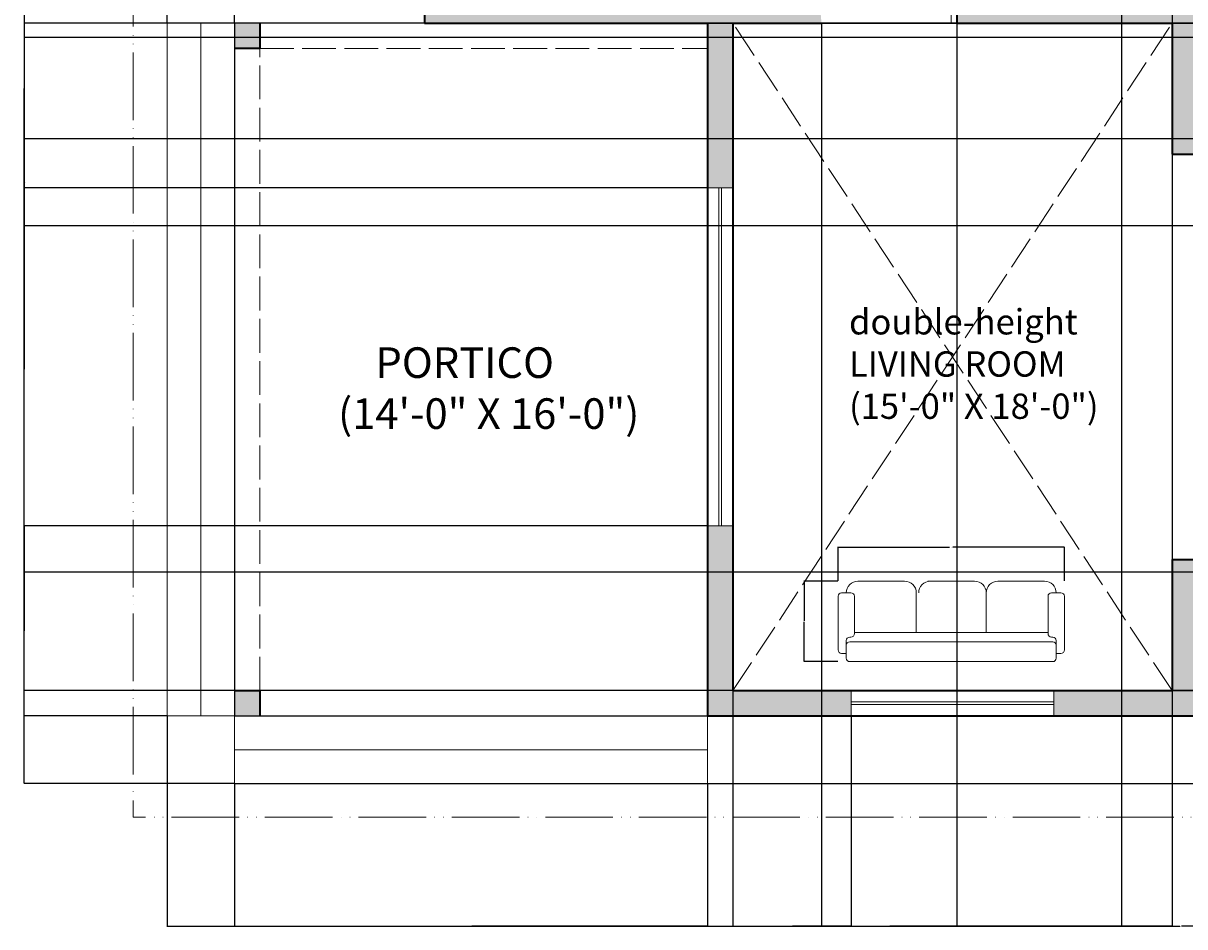
# Model space of a CAD drawing. Units: inches. Extents: x 2847 to 3693, y 1516 to 2098.
# Tile 1 of 6: x 2847 to 3259, y 1516 to 1837. Entities that reach past the tile are written whole.
import ezdxf

# ---------------------------------------------------------------- set-up
doc = ezdxf.new("R2010")
doc.units = ezdxf.units.IN
doc.linetypes.add('ACAD_ISO02W100', pattern=[15, 12, -3])
doc.linetypes.add('ACAD_ISO05W100', pattern=[33, 24, -3, 0, -3, 0, -3])
for name, color, linetype, lineweight in [('A-ANNO-DIMS', 2, 'Continuous', 18), ('A-AREA-IDEN', 7, 'Continuous', 18), ('A-COLS', 7, 'Continuous', 35), ('A-DOOR', 3, 'Continuous', 18), ('A-FLOR', 7, 'Continuous', 25), ('A-FLOR-OVHD', 8, 'ACAD_ISO02W100', 13), ('A-FLOR-STRS', 7, 'Continuous', 18), ('A-FURN', 8, 'Continuous', 18), ('A-GLAZ', 4, 'Continuous', 18), ('A-WALL', 7, 'Continuous', 35), ('C-PROP', 7, 'ACAD_ISO05W100', 18)]:
    doc.layers.add(name, color=color, linetype=linetype, lineweight=lineweight)
doc.layers.add('A-WALL-PATT', color=251, linetype='Continuous', lineweight=13, true_color=0x636466)
doc.styles.get("Standard").update_dxf_attribs({"font": 'arial.ttf'})
doc.dimstyles.get("Standard").update_dxf_attribs({"dimtxt": 0.18, "dimasz": 0.18, "dimexe": 0.18, "dimexo": 0.0625, "dimgap": 0.09, "dimtad": 0, "dimtih": 1, "dimtoh": 1, "dimdec": 4, "dimzin": 0, "dimdsep": 46, "dimtxsty": 'Standard', "dimcen": 0.09, "dimadec": 0, "dimazin": 0, "dimtfac": 1, "dimtdec": 4, "dimtofl": 0, "dimtmove": 0, "dimatfit": 3, "dimfxl": 1, "dimtolj": 1, "dimtzin": 0, "dimarcsym": 0})

# ---------------------------------------------------------------- blocks, each defined once
blk = doc.blocks.new('A$C115861F8')
for p, q in [((0.0679, 0.6013), (0.0291, 0.6013)), ((0.0679, 0.6401), (0.0679, 0.6013)), ((0.0679, 0.5334), (0.0679, 0.6013)), ((1.7846, 0.6692), (0.097, 0.6692)), ((1.8136, 0.6401), (1.8136, 0.6013)), ((1.8136, 0.6013), (1.8524, 0.6013)), ((1.8136, 0.5334), (1.8136, 0.6013)), ((0, 0.5722), (0, 0.1261)), ((0.0679, 0.4946), (0.0679, 0.5431)), ((1.7846, 0.5043), (0.097, 0.5043)), ((1.8136, 0.4946), (1.8136, 0.5431)), ((1.8815, 0.5722), (1.8815, 0.1261)), ((0.1067, 0.4655), (0.097, 0.4655)), ((0.1358, 0.1261), (0.1358, 0.4364)), ((1.7458, 0.4267), (0.1358, 0.4267)), ((0.6498, 0.097), (0.6498, 0.4267)), ((1.2317, 0.097), (1.2317, 0.4267)), ((1.7458, 0.1261), (1.7458, 0.4364)), ((1.7749, 0.4655), (1.7846, 0.4655)), ((0.0291, 0.097), (0.1067, 0.097)), ((1.8524, 0.097), (1.7749, 0.097)), ((0.1649, 0), (0.5528, 0)), ((1.1347, 0), (0.7468, 0)), ((1.3287, 0), (1.7167, 0))]:
    blk.add_line(p, q)
for centre, radius, start, end in [((0.0291, 0.5722), 0.0291, 90, 180), ((0.097, 0.6401), 0.0291, 90, 180), ((1.7846, 0.6401), 0.0291, 0, 90), ((1.8524, 0.5722), 0.0291, 0, 90), ((0.097, 0.5334), 0.0291, 180, 270), ((0.097, 0.4946), 0.0291, 180, 270), ((1.7846, 0.5334), 0.0291, 270, 0), ((1.7846, 0.4946), 0.0291, 270, 0), ((0.1067, 0.4364), 0.0291, 0, 90), ((1.7749, 0.4364), 0.0291, 90, 180), ((0.0291, 0.1261), 0.0291, 180, 270), ((0.1649, 0.097), 0.097, 180, 270), ((0.1067, 0.1261), 0.0291, 270, 0), ((0.5528, 0.097), 0.097, 270, 0), ((0.7468, 0.097), 0.097, 180, 270), ((1.1147, 0.097), 0.097, 270, 0), ((1.3287, 0.097), 0.097, 180, 270), ((1.7167, 0.097), 0.097, 270, 0), ((1.7749, 0.1261), 0.0291, 180, 270), ((1.8524, 0.1261), 0.0291, 270, 0)]:
    blk.add_arc(centre, radius, start, end)
blk = doc.blocks.new('WIN-GLAZ-72IN')
for p, q in [((0, 1), (72, 1)), ((0, 0), (72, 0))]:
    blk.add_line(p, q)
blk = doc.blocks.new('*D25')
at = {"layer": 'A-ANNO-DIMS', "color": 0, "lineweight": -2, "transparency": 16777216}
for p, q in [((3136.22, 1639.04), (3136.22, 1651.21)), ((3136.4, 1651.03), (3175.81, 1651.03)), ((3216.4, 1651.03), (3177, 1651.03)), ((3216.58, 1639.04), (3216.58, 1651.21))]:
    blk.add_line(p, q, dxfattribs=at)
at = {"layer": 'A-ANNO-DIMS', "color": 0, "transparency": 16777216}
for points in [[(3136.4, 1651.06), (3136.4, 1651), (3136.22, 1651.03)], [(3216.4, 1651.06), (3216.4, 1651), (3216.58, 1651.03)]]:
    blk.add_solid(points, dxfattribs=at)
at = {"layer": 'Defpoints', "color": 0, "transparency": 16777216}
for p in [(3136.22, 1651.03), (3136.22, 1638.98), (3216.58, 1638.98)]:
    blk.add_point(p, dxfattribs=at)
at = {"layer": 'A-ANNO-DIMS', "color": 0, "transparency": 16777216, "insert": (3176.4, 1651.03), "char_height": 0.18, "attachment_point": 5}
blk.add_mtext('\\A1;SOFA 80', dxfattribs=at)
blk = doc.blocks.new('*D26')
at = {"layer": 'A-ANNO-DIMS', "color": 0, "lineweight": -2, "transparency": 16777216}
for p, q in [((3136.16, 1638.98), (3123.98, 1638.98)), ((3124.16, 1638.8), (3124.16, 1624.87)), ((3124.16, 1610.58), (3124.16, 1624.51)), ((3136.16, 1610.4), (3123.98, 1610.4))]:
    blk.add_line(p, q, dxfattribs=at)
at = {"layer": 'A-ANNO-DIMS', "color": 0, "transparency": 16777216}
for points in [[(3124.13, 1638.8), (3124.19, 1638.8), (3124.16, 1638.98)], [(3124.13, 1610.58), (3124.19, 1610.58), (3124.16, 1610.4)]]:
    blk.add_solid(points, dxfattribs=at)
at = {"layer": 'Defpoints', "color": 0, "transparency": 16777216}
for p in [(3136.22, 1638.98), (3124.16, 1610.4), (3136.22, 1610.4)]:
    blk.add_point(p, dxfattribs=at)
at = {"layer": 'A-ANNO-DIMS', "color": 0, "transparency": 16777216, "insert": (3124.16, 1624.69), "char_height": 0.18, "attachment_point": 5}
blk.add_mtext('\\A1;29', dxfattribs=at)
blk = doc.blocks.new('*D37')
at = {"layer": 'A-ANNO-DIMS', "color": 0, "lineweight": -2, "transparency": 16777216}
for p, q in [((3617.85, 1765.06), (3617.85, 1516.24)), ((2897.85, 1591.06), (2897.85, 1516.24)), ((2898.03, 1516.42), (3257.56, 1516.42)), ((3617.67, 1516.42), (3258.13, 1516.42))]:
    blk.add_line(p, q, dxfattribs=at)
at = {"layer": 'A-ANNO-DIMS', "color": 0, "transparency": 16777216}
for points in [[(2898.03, 1516.45), (2898.03, 1516.39), (2897.85, 1516.42)], [(3617.67, 1516.45), (3617.67, 1516.39), (3617.85, 1516.42)]]:
    blk.add_solid(points, dxfattribs=at)
at = {"layer": 'Defpoints', "color": 0, "transparency": 16777216}
for p in [(3617.85, 1765.12), (2897.85, 1591.12), (3617.85, 1516.42)]:
    blk.add_point(p, dxfattribs=at)
at = {"layer": 'A-ANNO-DIMS', "color": 0, "transparency": 16777216, "insert": (3257.85, 1516.42), "char_height": 0.18, "attachment_point": 5}
blk.add_mtext('\\A1;720', dxfattribs=at)
blk = doc.blocks.new('*D38')
at = {"layer": 'A-ANNO-DIMS', "color": 0, "lineweight": -2, "transparency": 16777216}
for p, q in [((2989.283202, 2011.118004), (2846.965702, 2011.118004)), ((2847.145702, 2010.938004), (2847.145702, 1789.298004)), ((2847.145702, 1567.298004), (2847.145702, 1788.938004)), ((2921.783202, 1567.118004), (2846.965702, 1567.118004))]:
    blk.add_line(p, q, dxfattribs=at)
at = {"layer": 'A-ANNO-DIMS', "color": 0, "transparency": 16777216}
for points in [[(2847.115702, 2010.938004), (2847.175702, 2010.938004), (2847.145702, 2011.118004)], [(2847.115702, 1567.298004), (2847.175702, 1567.298004), (2847.145702, 1567.118004)]]:
    blk.add_solid(points, dxfattribs=at)
at = {"layer": 'Defpoints', "color": 0, "transparency": 16777216}
for p in [(2847.145702, 2011.118004), (2989.345702, 2011.118004), (2921.845702, 1567.118004)]:
    blk.add_point(p, dxfattribs=at)
at = {"layer": 'A-ANNO-DIMS', "color": 0, "transparency": 16777216, "insert": (2847.145702, 1789.118004), "char_height": 0.18, "attachment_point": 5}
blk.add_mtext('\\A1;444', dxfattribs=at)
blk = doc.blocks.new('*D43')
at = {"layer": 'A-ANNO-DIMS', "color": 0, "lineweight": -2, "transparency": 16777216}
for p, q in [((2921.85, 1567.06), (2921.85, 1516.24)), ((3089.85, 1567.06), (3089.85, 1516.24)), ((2922.03, 1516.42), (3005.57, 1516.42)), ((3089.67, 1516.42), (3006.13, 1516.42))]:
    blk.add_line(p, q, dxfattribs=at)
at = {"layer": 'A-ANNO-DIMS', "color": 0, "transparency": 16777216}
for points in [[(2922.03, 1516.45), (2922.03, 1516.39), (2921.85, 1516.42)], [(3089.67, 1516.45), (3089.67, 1516.39), (3089.85, 1516.42)]]:
    blk.add_solid(points, dxfattribs=at)
at = {"layer": 'Defpoints', "color": 0, "transparency": 16777216}
for p in [(2921.85, 1567.12), (3089.85, 1567.12), (3089.85, 1516.42)]:
    blk.add_point(p, dxfattribs=at)
at = {"layer": 'A-ANNO-DIMS', "color": 0, "transparency": 16777216, "insert": (3005.85, 1516.42), "char_height": 0.18, "attachment_point": 5}
blk.add_mtext('\\A1;168', dxfattribs=at)
blk = doc.blocks.new('*D44')
at = {"layer": 'A-ANNO-DIMS', "color": 0, "lineweight": -2, "transparency": 16777216}
for p, q in [((2921.85, 1837.18), (2921.85, 2098)), ((2922.03, 2097.82), (2955.27, 2097.82)), ((2989.17, 2097.82), (2955.92, 2097.82)), ((2989.35, 1837.18), (2989.35, 2098))]:
    blk.add_line(p, q, dxfattribs=at)
at = {"layer": 'A-ANNO-DIMS', "color": 0, "transparency": 16777216}
for points in [[(2922.03, 2097.85), (2922.03, 2097.79), (2921.85, 2097.82)], [(2989.17, 2097.85), (2989.17, 2097.79), (2989.35, 2097.82)]]:
    blk.add_solid(points, dxfattribs=at)
at = {"layer": 'Defpoints', "color": 0, "transparency": 16777216}
for p in [(2989.35, 2097.82), (2921.85, 1837.12), (2989.35, 1837.12)]:
    blk.add_point(p, dxfattribs=at)
at = {"layer": 'A-ANNO-DIMS', "color": 0, "transparency": 16777216, "insert": (2955.6, 2097.82), "char_height": 0.18, "attachment_point": 5}
blk.add_mtext('\\A1;67.5', dxfattribs=at)
blk = doc.blocks.new('*D45')
at = {"layer": 'A-ANNO-DIMS', "color": 0, "lineweight": -2, "transparency": 16777216}
for p, q in [((3098.85, 1600.06), (3098.85, 1516.24)), ((3254.85, 1600.06), (3254.85, 1516.24)), ((3099.03, 1516.42), (3176.57, 1516.42)), ((3254.67, 1516.42), (3177.13, 1516.42))]:
    blk.add_line(p, q, dxfattribs=at)
at = {"layer": 'A-ANNO-DIMS', "color": 0, "transparency": 16777216}
for points in [[(3099.03, 1516.45), (3099.03, 1516.39), (3098.85, 1516.42)], [(3254.67, 1516.45), (3254.67, 1516.39), (3254.85, 1516.42)]]:
    blk.add_solid(points, dxfattribs=at)
at = {"layer": 'Defpoints', "color": 0, "transparency": 16777216}
for p in [(3098.85, 1600.12), (3254.85, 1600.12), (3254.85, 1516.42)]:
    blk.add_point(p, dxfattribs=at)
at = {"layer": 'A-ANNO-DIMS', "color": 0, "transparency": 16777216, "insert": (3176.85, 1516.42), "char_height": 0.18, "attachment_point": 5}
blk.add_mtext('\\A1;156', dxfattribs=at)
blk = doc.blocks.new('*D50')
at = {"layer": 'A-ANNO-DIMS', "color": 0, "lineweight": -2, "transparency": 16777216}
for p, q in [((2989.41, 2011.12), (3692.73, 2011.12)), ((3692.55, 2010.94), (3692.55, 1924.3)), ((3692.55, 1837.3), (3692.55, 1923.94)), ((2989.41, 1837.12), (3692.73, 1837.12))]:
    blk.add_line(p, q, dxfattribs=at)
at = {"layer": 'A-ANNO-DIMS', "color": 0, "transparency": 16777216}
for points in [[(3692.52, 2010.94), (3692.58, 2010.94), (3692.55, 2011.12)], [(3692.52, 1837.3), (3692.58, 1837.3), (3692.55, 1837.12)]]:
    blk.add_solid(points, dxfattribs=at)
at = {"layer": 'Defpoints', "color": 0, "transparency": 16777216}
for p in [(2989.35, 2011.12), (3692.55, 2011.12), (2989.35, 1837.12)]:
    blk.add_point(p, dxfattribs=at)
at = {"layer": 'A-ANNO-DIMS', "color": 0, "transparency": 16777216, "insert": (3692.55, 1924.12), "char_height": 0.18, "attachment_point": 5}
blk.add_mtext('\\A1;174', dxfattribs=at)
blk = doc.blocks.new('*D51')
at = {"layer": 'A-ANNO-DIMS', "color": 0, "lineweight": -2, "transparency": 16777216}
for p, q in [((2897.78, 1837.12), (2846.97, 1837.12)), ((2847.15, 1836.94), (2847.15, 1714.3)), ((2847.15, 1591.3), (2847.15, 1713.94)), ((2897.78, 1591.12), (2846.97, 1591.12))]:
    blk.add_line(p, q, dxfattribs=at)
at = {"layer": 'A-ANNO-DIMS', "color": 0, "transparency": 16777216}
for points in [[(2847.12, 1836.94), (2847.18, 1836.94), (2847.15, 1837.12)], [(2847.12, 1591.3), (2847.18, 1591.3), (2847.15, 1591.12)]]:
    blk.add_solid(points, dxfattribs=at)
at = {"layer": 'Defpoints', "color": 0, "transparency": 16777216}
for p in [(2847.15, 1837.12), (2897.85, 1837.12), (2897.85, 1591.12)]:
    blk.add_point(p, dxfattribs=at)
at = {"layer": 'A-ANNO-DIMS', "color": 0, "transparency": 16777216, "insert": (2847.15, 1714.12), "char_height": 0.18, "attachment_point": 5}
blk.add_mtext('\\A1;246', dxfattribs=at)
blk = doc.blocks.new('*D52')
at = {"layer": 'A-ANNO-DIMS', "color": 0, "lineweight": -2, "transparency": 16777216}
for p, q in [((3505.28, 1837.12), (2846.97, 1837.12)), ((2847.15, 1836.94), (2847.15, 1801.3)), ((2847.15, 1765.3), (2847.15, 1800.94)), ((3505.28, 1765.12), (2846.97, 1765.12))]:
    blk.add_line(p, q, dxfattribs=at)
at = {"layer": 'A-ANNO-DIMS', "color": 0, "transparency": 16777216}
for points in [[(2847.12, 1836.94), (2847.18, 1836.94), (2847.15, 1837.12)], [(2847.12, 1765.3), (2847.18, 1765.3), (2847.15, 1765.12)]]:
    blk.add_solid(points, dxfattribs=at)
at = {"layer": 'Defpoints', "color": 0, "transparency": 16777216}
for p in [(2847.15, 1837.12), (3505.35, 1837.12), (3505.35, 1765.12)]:
    blk.add_point(p, dxfattribs=at)
at = {"layer": 'A-ANNO-DIMS', "color": 0, "transparency": 16777216, "insert": (2847.15, 1801.12), "char_height": 0.18, "attachment_point": 5}
blk.add_mtext('\\A1;72', dxfattribs=at)
blk = doc.blocks.new('*D54')
at = {"layer": 'A-ANNO-DIMS', "color": 0, "lineweight": -2, "transparency": 16777216}
for p, q in [((3130.35, 1837.06), (3130.35, 1516.24)), ((3178.35, 1837.06), (3178.35, 1516.24)), ((3130.53, 1516.42), (3154.12, 1516.42)), ((3178.17, 1516.42), (3154.57, 1516.42))]:
    blk.add_line(p, q, dxfattribs=at)
at = {"layer": 'A-ANNO-DIMS', "color": 0, "transparency": 16777216}
for points in [[(3130.53, 1516.45), (3130.53, 1516.39), (3130.35, 1516.42)], [(3178.17, 1516.45), (3178.17, 1516.39), (3178.35, 1516.42)]]:
    blk.add_solid(points, dxfattribs=at)
at = {"layer": 'Defpoints', "color": 0, "transparency": 16777216}
for p in [(3130.35, 1837.12), (3178.35, 1837.12), (3178.35, 1516.42)]:
    blk.add_point(p, dxfattribs=at)
at = {"layer": 'A-ANNO-DIMS', "color": 0, "transparency": 16777216, "insert": (3154.35, 1516.42), "char_height": 0.18, "attachment_point": 5}
blk.add_mtext('\\A1;48', dxfattribs=at)
blk = doc.blocks.new('*D58')
at = {"layer": 'A-ANNO-DIMS', "color": 0, "lineweight": -2, "transparency": 16777216}
for p, q in [((3089.78, 1778.62), (2846.97, 1778.62)), ((2847.15, 1778.44), (2847.15, 1718.8)), ((2847.15, 1658.8), (2847.15, 1718.44)), ((3089.78, 1658.62), (2846.97, 1658.62))]:
    blk.add_line(p, q, dxfattribs=at)
at = {"layer": 'A-ANNO-DIMS', "color": 0, "transparency": 16777216}
for points in [[(2847.12, 1778.44), (2847.18, 1778.44), (2847.15, 1778.62)], [(2847.12, 1658.8), (2847.18, 1658.8), (2847.15, 1658.62)]]:
    blk.add_solid(points, dxfattribs=at)
at = {"layer": 'Defpoints', "color": 0, "transparency": 16777216}
for p in [(2847.15, 1778.62), (3089.85, 1778.62), (3089.85, 1658.62)]:
    blk.add_point(p, dxfattribs=at)
at = {"layer": 'A-ANNO-DIMS', "color": 0, "transparency": 16777216, "insert": (2847.15, 1718.62), "char_height": 0.18, "attachment_point": 5}
blk.add_mtext('\\A1;120', dxfattribs=at)
blk = doc.blocks.new('*D59')
at = {"layer": 'A-ANNO-DIMS', "color": 0, "lineweight": -2, "transparency": 16777216}
for p, q in [((3098.85, 1600.06), (3098.85, 1516.24)), ((3140.85, 1591.06), (3140.85, 1516.24)), ((3099.03, 1516.42), (3119.62, 1516.42)), ((3140.67, 1516.42), (3120.07, 1516.42))]:
    blk.add_line(p, q, dxfattribs=at)
at = {"layer": 'A-ANNO-DIMS', "color": 0, "transparency": 16777216}
for points in [[(3099.03, 1516.45), (3099.03, 1516.39), (3098.85, 1516.42)], [(3140.67, 1516.45), (3140.67, 1516.39), (3140.85, 1516.42)]]:
    blk.add_solid(points, dxfattribs=at)
at = {"layer": 'Defpoints', "color": 0, "transparency": 16777216}
for p in [(3098.85, 1600.12), (3140.85, 1591.12), (3098.85, 1516.42)]:
    blk.add_point(p, dxfattribs=at)
at = {"layer": 'A-ANNO-DIMS', "color": 0, "transparency": 16777216, "insert": (3119.85, 1516.42), "char_height": 0.18, "attachment_point": 5}
blk.add_mtext('\\A1;42', dxfattribs=at)
blk = doc.blocks.new('*D63')
at = {"layer": 'A-ANNO-DIMS', "color": 0, "lineweight": -2, "transparency": 16777216}
for p, q in [((2897.85, 1837.18), (2897.85, 2098)), ((2898.03, 2097.82), (2909.63, 2097.82)), ((2921.67, 2097.82), (2910.07, 2097.82)), ((2921.85, 1837.18), (2921.85, 2098))]:
    blk.add_line(p, q, dxfattribs=at)
at = {"layer": 'A-ANNO-DIMS', "color": 0, "transparency": 16777216}
for points in [[(2898.03, 2097.85), (2898.03, 2097.79), (2897.85, 2097.82)], [(2921.67, 2097.85), (2921.67, 2097.79), (2921.85, 2097.82)]]:
    blk.add_solid(points, dxfattribs=at)
at = {"layer": 'Defpoints', "color": 0, "transparency": 16777216}
for p in [(2921.85, 2097.82), (2897.85, 1837.12), (2921.85, 1837.12)]:
    blk.add_point(p, dxfattribs=at)
at = {"layer": 'A-ANNO-DIMS', "color": 0, "transparency": 16777216, "insert": (2909.85, 2097.82), "char_height": 0.18, "attachment_point": 5}
blk.add_mtext('\\A1;24', dxfattribs=at)
blk = doc.blocks.new('*D64')
at = {"layer": 'A-ANNO-DIMS', "color": 0, "lineweight": -2, "transparency": 16777216}
for p, q in [((2921.91, 1591.12), (3692.73, 1591.12)), ((3692.55, 1590.94), (3692.55, 1579.3)), ((3692.55, 1567.3), (3692.55, 1578.94)), ((2921.91, 1567.12), (3692.73, 1567.12))]:
    blk.add_line(p, q, dxfattribs=at)
at = {"layer": 'A-ANNO-DIMS', "color": 0, "transparency": 16777216}
for points in [[(3692.52, 1590.94), (3692.58, 1590.94), (3692.55, 1591.12)], [(3692.52, 1567.3), (3692.58, 1567.3), (3692.55, 1567.12)]]:
    blk.add_solid(points, dxfattribs=at)
at = {"layer": 'Defpoints', "color": 0, "transparency": 16777216}
for p in [(2921.85, 1591.12), (3692.55, 1591.12), (2921.85, 1567.12)]:
    blk.add_point(p, dxfattribs=at)
at = {"layer": 'A-ANNO-DIMS', "color": 0, "transparency": 16777216, "insert": (3692.55, 1579.12), "char_height": 0.18, "attachment_point": 5}
blk.add_mtext('\\A1;24', dxfattribs=at)
blk = doc.blocks.new('*D69')
at = {"layer": 'A-ANNO-DIMS', "color": 0, "lineweight": -2, "transparency": 16777216}
for p, q in [((3089.78, 1658.62), (2846.97, 1658.62)), ((2847.15, 1658.44), (2847.15, 1629.55)), ((2847.15, 1600.3), (2847.15, 1629.19)), ((3089.78, 1600.12), (2846.97, 1600.12))]:
    blk.add_line(p, q, dxfattribs=at)
at = {"layer": 'A-ANNO-DIMS', "color": 0, "transparency": 16777216}
for points in [[(2847.12, 1658.44), (2847.18, 1658.44), (2847.15, 1658.62)], [(2847.12, 1600.3), (2847.18, 1600.3), (2847.15, 1600.12)]]:
    blk.add_solid(points, dxfattribs=at)
at = {"layer": 'Defpoints', "color": 0, "transparency": 16777216}
for p in [(2847.15, 1658.62), (3089.85, 1658.62), (3089.85, 1600.12)]:
    blk.add_point(p, dxfattribs=at)
at = {"layer": 'A-ANNO-DIMS', "color": 0, "transparency": 16777216, "insert": (2847.15, 1629.37), "char_height": 0.18, "attachment_point": 5}
blk.add_mtext('\\A1;58.5', dxfattribs=at)
blk = doc.blocks.new('*D71')
at = {"layer": 'A-ANNO-DIMS', "color": 0, "lineweight": -2, "transparency": 16777216}
for p, q in [((3254.91, 1790.62), (3692.73, 1790.62)), ((3692.55, 1790.44), (3692.55, 1718.8)), ((3692.55, 1646.8), (3692.55, 1718.44)), ((3254.91, 1646.62), (3692.73, 1646.62))]:
    blk.add_line(p, q, dxfattribs=at)
at = {"layer": 'A-ANNO-DIMS', "color": 0, "transparency": 16777216}
for points in [[(3692.52, 1790.44), (3692.58, 1790.44), (3692.55, 1790.62)], [(3692.52, 1646.8), (3692.58, 1646.8), (3692.55, 1646.62)]]:
    blk.add_solid(points, dxfattribs=at)
at = {"layer": 'Defpoints', "color": 0, "transparency": 16777216}
for p in [(3254.85, 1790.62), (3692.55, 1790.62), (3254.85, 1646.62)]:
    blk.add_point(p, dxfattribs=at)
at = {"layer": 'A-ANNO-DIMS', "color": 0, "transparency": 16777216, "insert": (3692.55, 1718.62), "char_height": 0.18, "attachment_point": 5}
blk.add_mtext('\\A1;144', dxfattribs=at)
blk = doc.blocks.new('*D72')
at = {"layer": 'A-ANNO-DIMS', "color": 0, "lineweight": -2, "transparency": 16777216}
for p, q in [((3254.91, 1646.62), (3692.73, 1646.62)), ((3692.55, 1646.44), (3692.55, 1623.55)), ((3692.55, 1600.3), (3692.55, 1623.19)), ((3254.91, 1600.12), (3692.73, 1600.12))]:
    blk.add_line(p, q, dxfattribs=at)
at = {"layer": 'A-ANNO-DIMS', "color": 0, "transparency": 16777216}
for points in [[(3692.52, 1646.44), (3692.58, 1646.44), (3692.55, 1646.62)], [(3692.52, 1600.3), (3692.58, 1600.3), (3692.55, 1600.12)]]:
    blk.add_solid(points, dxfattribs=at)
at = {"layer": 'Defpoints', "color": 0, "transparency": 16777216}
for p in [(3254.85, 1646.62), (3692.55, 1646.62), (3254.85, 1600.12)]:
    blk.add_point(p, dxfattribs=at)
at = {"layer": 'A-ANNO-DIMS', "color": 0, "transparency": 16777216, "insert": (3692.55, 1623.37), "char_height": 0.18, "attachment_point": 5}
blk.add_mtext('\\A1;46.5', dxfattribs=at)
blk = doc.blocks.new('*D75')
at = {"layer": 'A-ANNO-DIMS', "color": 0, "lineweight": -2, "transparency": 16777216}
for p, q in [((3236.85, 2002.06), (3236.85, 1516.24)), ((3254.85, 2002.06), (3254.85, 1516.24)), ((3237.03, 1516.42), (3245.64, 1516.42)), ((3254.67, 1516.42), (3246.06, 1516.42))]:
    blk.add_line(p, q, dxfattribs=at)
at = {"layer": 'A-ANNO-DIMS', "color": 0, "transparency": 16777216}
for points in [[(3237.03, 1516.45), (3237.03, 1516.39), (3236.85, 1516.42)], [(3254.67, 1516.45), (3254.67, 1516.39), (3254.85, 1516.42)]]:
    blk.add_solid(points, dxfattribs=at)
at = {"layer": 'Defpoints', "color": 0, "transparency": 16777216}
for p in [(3236.85, 2002.12), (3254.85, 2002.12), (3254.85, 1516.42)]:
    blk.add_point(p, dxfattribs=at)
at = {"layer": 'A-ANNO-DIMS', "color": 0, "transparency": 16777216, "insert": (3245.85, 1516.42), "char_height": 0.18, "attachment_point": 5}
blk.add_mtext('\\A1;18', dxfattribs=at)
blk = doc.blocks.new('*D76')
at = {"layer": 'A-ANNO-DIMS', "color": 0, "lineweight": -2, "transparency": 16777216}
for p, q in [((3584.78, 1642.12), (2846.97, 1642.12)), ((2847.15, 1641.94), (2847.15, 1621.3)), ((2847.15, 1600.3), (2847.15, 1620.94)), ((3584.78, 1600.12), (2846.97, 1600.12))]:
    blk.add_line(p, q, dxfattribs=at)
at = {"layer": 'A-ANNO-DIMS', "color": 0, "transparency": 16777216}
for points in [[(2847.12, 1641.94), (2847.18, 1641.94), (2847.15, 1642.12)], [(2847.12, 1600.3), (2847.18, 1600.3), (2847.15, 1600.12)]]:
    blk.add_solid(points, dxfattribs=at)
at = {"layer": 'Defpoints', "color": 0, "transparency": 16777216}
for p in [(2847.15, 1642.12), (3584.85, 1642.12), (3584.85, 1600.12)]:
    blk.add_point(p, dxfattribs=at)
at = {"layer": 'A-ANNO-DIMS', "color": 0, "transparency": 16777216, "insert": (2847.15, 1621.12), "char_height": 0.18, "attachment_point": 5}
blk.add_mtext('\\A1;42', dxfattribs=at)
blk = doc.blocks.new('*D77')
at = {"layer": 'A-ANNO-DIMS', "color": 0, "lineweight": -2, "transparency": 16777216}
for p, q in [((3584.78, 1832.08), (2846.97, 1832.08)), ((2847.15, 1831.9), (2847.15, 1814.27)), ((2847.15, 1796.26), (2847.15, 1813.9)), ((3584.78, 1796.08), (2846.97, 1796.08))]:
    blk.add_line(p, q, dxfattribs=at)
at = {"layer": 'A-ANNO-DIMS', "color": 0, "transparency": 16777216}
for points in [[(2847.12, 1831.9), (2847.18, 1831.9), (2847.15, 1832.08)], [(2847.12, 1796.26), (2847.18, 1796.26), (2847.15, 1796.08)]]:
    blk.add_solid(points, dxfattribs=at)
at = {"layer": 'Defpoints', "color": 0, "transparency": 16777216}
for p in [(2847.15, 1832.08), (3584.85, 1832.08), (3584.85, 1796.08)]:
    blk.add_point(p, dxfattribs=at)
at = {"layer": 'A-ANNO-DIMS', "color": 0, "transparency": 16777216, "insert": (2847.15, 1814.08), "char_height": 0.18, "attachment_point": 5}
blk.add_mtext('\\A1;36', dxfattribs=at)
blk = doc.blocks.new('*D78')
at = {"layer": 'A-ANNO-DIMS', "color": 0, "lineweight": -2, "transparency": 16777216}
for p, q in [((3584.78, 1796.08), (2846.97, 1796.08)), ((2847.15, 1795.9), (2847.15, 1780.78)), ((2847.15, 1765.3), (2847.15, 1780.42)), ((3584.78, 1765.12), (2846.97, 1765.12))]:
    blk.add_line(p, q, dxfattribs=at)
at = {"layer": 'A-ANNO-DIMS', "color": 0, "transparency": 16777216}
for points in [[(2847.12, 1795.9), (2847.18, 1795.9), (2847.15, 1796.08)], [(2847.12, 1765.3), (2847.18, 1765.3), (2847.15, 1765.12)]]:
    blk.add_solid(points, dxfattribs=at)
at = {"layer": 'Defpoints', "color": 0, "transparency": 16777216}
for p in [(2847.15, 1796.08), (3584.85, 1796.08), (3584.85, 1765.12)]:
    blk.add_point(p, dxfattribs=at)
at = {"layer": 'A-ANNO-DIMS', "color": 0, "transparency": 16777216, "insert": (2847.15, 1780.6), "char_height": 0.18, "attachment_point": 5}
blk.add_mtext('\\A1;30.965', dxfattribs=at)

msp = doc.modelspace()

# ---------------------------------------------------------------- hatches: boundary and pattern name
at = {"layer": 'A-WALL-PATT'}
h = msp.add_hatch(color=256, dxfattribs=at)
h.dxf.hatch_style = 1
h.paths.add_polyline_path([(2998.3457, 2002.118), (3178.3457, 2002.118), (3178.3457, 1944.368, -0.0341147), (3182.8457, 1944.4698), (3182.8457, 2002.118), (3200.8457, 2002.118), (3200.8457, 2011.118), (2989.3457, 2011.118), (2989.3457, 1960.118), (2998.3457, 1960.118)])
h.paths.add_polyline_path([(2998.3457, 1888.118), (2989.3457, 1888.118), (2989.3457, 1837.118), (3089.8457, 1837.118), (3089.8457, 1778.618), (3098.8457, 1778.618), (3098.8457, 1837.118), (3130.3457, 1837.118, -0.05293254), (3130.1282, 1846.118), (2998.3457, 1846.118)])
h.paths.add_polyline_path([(3263.8457, 2002.118), (3311.8457, 2002.118), (3311.8457, 2011.118), (3263.8457, 2011.118), (3236.8457, 2011.118), (3236.8457, 2002.118), (3254.8457, 2002.118), (3254.8457, 1908.368), (3182.8457, 1908.368), (3178.3457, 1908.368), (3178.3457, 1886.993), (3182.8457, 1886.993), (3182.8457, 1903.868), (3254.8457, 1903.868), (3254.8457, 1846.118), (3182.8457, 1846.118), (3182.8457, 1850.993), (3178.3457, 1850.993), (3178.3457, 1837.118), (3254.8457, 1837.118), (3254.8457, 1790.618), (3263.8457, 1790.618), (3263.8457, 1837.118)])
h.paths.add_polyline_path([(2930.8457, 1837.118), (2921.8457, 1837.118), (2921.8457, 1828.118), (2930.8457, 1828.118)])
h.paths.add_polyline_path([(2930.8457, 1600.118), (2921.8457, 1600.118), (2921.8457, 1591.118), (2930.8457, 1591.118)])
h.paths.add_polyline_path([(3098.8457, 1658.618), (3089.8457, 1658.618), (3089.8457, 1591.118), (3140.8457, 1591.118), (3140.8457, 1600.118), (3098.8457, 1600.118)])
h.paths.add_polyline_path([(3305.8457, 1600.118), (3263.8457, 1600.118), (3263.8457, 1646.618), (3254.8457, 1646.618), (3254.8457, 1600.118), (3212.8457, 1600.118), (3212.8457, 1591.118), (3254.8457, 1591.118), (3305.8457, 1591.118)])
h.paths.add_polyline_path([(3470.8457, 1600.118), (3428.8457, 1600.118), (3428.8457, 1756.118), (3430.26, 1756.118), (3430.26, 1765.118), (3428.8457, 1765.118), (3419.8457, 1765.118), (3419.8457, 1600.118), (3377.8457, 1600.118), (3377.8457, 1591.118), (3470.8457, 1591.118)])
h.paths.add_polyline_path([(3593.8457, 1642.118), (3584.8457, 1642.118), (3584.8457, 1600.118), (3542.8457, 1600.118), (3542.8457, 1591.118), (3593.8457, 1591.118)])
h.paths.add_polyline_path([(3593.8457, 1796.083), (3584.8457, 1796.083), (3584.8457, 1765.118), (3505.3457, 1765.118), (3505.3457, 1837.118), (3584.8457, 1837.118), (3584.8457, 1832.083), (3593.8457, 1832.083), (3593.8457, 1837.118), (3593.8457, 1924.118), (3584.8457, 1924.118), (3584.8457, 1846.118), (3478.26, 1846.118), (3478.26, 1837.118), (3500.8457, 1837.118), (3500.8457, 1765.118), (3478.26, 1765.118, -0.03536449), (3478.26, 1758.7816), (3478.26, 1756.118), (3584.8457, 1756.118), (3584.8457, 1714.118), (3593.8457, 1714.118)])
h.paths.add_polyline_path([(3593.8457, 2011.118), (3536.8457, 2011.118), (3536.8457, 2002.118), (3584.8457, 2002.118), (3584.8457, 1960.118), (3593.8457, 1960.118)])
h.paths.add_polyline_path([(3476.8457, 2011.118), (3371.8457, 2011.118), (3371.8457, 2002.118), (3419.8457, 2002.118), (3419.8457, 1837.118), (3428.8457, 1837.118), (3430.26, 1837.118), (3430.26, 1846.118), (3428.8457, 1846.118), (3428.8457, 2002.118), (3476.8457, 2002.118)])

# ---------------------------------------------------------------- linework, layer by layer
at = {"layer": 'A-COLS'}
for p, q in [((2930.8457, 1837.118), (2930.8457, 1828.118)), ((2930.8457, 1828.118), (2921.8457, 1828.118)), ((2921.8457, 1600.118), (2930.8457, 1600.118)), ((2930.8457, 1600.118), (2930.8457, 1591.118))]:
    msp.add_line(p, q, dxfattribs=at)
at = {"layer": 'A-DOOR'}
for p, q in [((3176.3457, 1885.118), (3176.3457, 1837.118)), ((3178.3457, 1837.118), (3178.3457, 1885.118)), ((3176.3457, 1837.118), (3178.3457, 1837.118))]:
    msp.add_line(p, q, dxfattribs=at)
at = {"layer": 'A-FLOR'}
for p, q in [((2921.8457, 1837.118), (2921.8457, 1591.118)), ((2989.3457, 1837.118), (2921.8457, 1837.118)), ((2921.8457, 1591.118), (3089.8457, 1591.118))]:
    msp.add_line(p, q, dxfattribs=at)
at = {"layer": 'A-FLOR-OVHD'}
for p, q in [((3098.8457, 1600.118), (3254.8457, 1837.118)), ((3254.8457, 1600.118), (3098.8457, 1837.118)), ((2930.8457, 1600.118), (2930.8457, 1828.118)), ((2930.8457, 1828.118), (3089.8457, 1828.118)), ((3254.8457, 1790.618), (3254.8457, 1646.618)), ((2930.8457, 1600.118), (3089.8457, 1600.118))]:
    msp.add_line(p, q, dxfattribs=at)
at = {"layer": 'A-FLOR-STRS'}
for p, q in [((2897.8457, 1837.118), (2897.8457, 1591.118)), ((2897.8457, 1837.118), (2921.8457, 1837.118)), ((2909.8457, 1837.118), (2909.8457, 1591.118)), ((2897.8457, 1591.118), (2921.8457, 1591.118)), ((2921.8457, 1567.118), (2921.8457, 1591.118)), ((3089.8457, 1591.118), (3089.8457, 1567.118)), ((3089.8457, 1579.118), (2921.8457, 1579.118)), ((3089.8457, 1567.118), (2921.8457, 1567.118))]:
    msp.add_line(p, q, dxfattribs=at)
at = {"layer": 'A-GLAZ'}
for p, q in [((3098.8457, 1778.618), (3089.8457, 1778.618)), ((3093.8457, 1658.618), (3093.8457, 1778.618)), ((3094.8457, 1658.618), (3094.8457, 1778.618)), ((3098.8457, 1658.618), (3089.8457, 1658.618)), ((3140.8457, 1600.118), (3140.8457, 1591.118)), ((3212.8457, 1600.118), (3212.8457, 1591.118))]:
    msp.add_line(p, q, dxfattribs=at)
at = {"layer": 'A-WALL'}
for p, q in [((2989.3457, 2011.118), (2989.3457, 1837.118)), ((3178.3457, 1846.118), (3178.3457, 1837.118)), ((2989.3457, 1837.118), (3089.8457, 1837.118)), ((3089.8457, 1837.118), (3089.8457, 1591.118)), ((3098.8457, 1837.118), (3098.8457, 1600.118)), ((3098.8457, 1837.118), (3130.3457, 1837.118)), ((3178.3457, 1837.118), (3254.8457, 1837.118)), ((3254.8457, 1837.118), (3254.8457, 1790.618)), ((3254.8457, 1790.618), (3263.8457, 1790.618)), ((3254.8457, 1646.618), (3263.8457, 1646.618)), ((3254.8457, 1646.618), (3254.8457, 1600.118)), ((3098.8457, 1600.118), (3254.8457, 1600.118)), ((3089.8457, 1591.118), (3254.8457, 1591.118)), ((3254.8457, 1591.118), (3593.8457, 1591.118))]:
    msp.add_line(p, q, dxfattribs=at)
at = {"layer": 'C-PROP'}
for p in [(2885.8457, 2059.118), (3653.8457, 1555.118)]:
    msp.add_line(p, (2885.8457, 1555.118), dxfattribs=at)

# ---------------------------------------------------------------- block references
at = {"layer": 'A-FURN', "xscale": 42.71149854958664, "yscale": 42.71149854958664, "zscale": 42.71149854958664, "rotation": 180}
msp.add_blockref('A$C115861F8', (3216.5826, 1638.98), dxfattribs=at)
at = {"layer": 'A-GLAZ'}
msp.add_blockref('WIN-GLAZ-72IN', (3140.846, 1595.118), dxfattribs=at)

# ---------------------------------------------------------------- texts
at = {"layer": 'A-AREA-IDEN', "attachment_point": 1}
for s, width, gutter_width, insert, char_height in [('double-height\\PLIVING ROOM \\P(15\'-0" X 18\'-0")', 240.035183, 44.958, (3140.1006, 1735.5897), 8.991601), ('    PORTICO\\P(14\'-0" X 16\'-0")', 289.838452, 54.286, (2958.6045, 1722.015), 10.857207)]:
    msp.add_mtext_dynamic_manual_height_columns(s, width=width, gutter_width=gutter_width, heights=[0], dxfattribs=dict(at, insert=insert, char_height=char_height))

# ---------------------------------------------------------------- dimensions: what is measured, and where the dimension line sits
at = {"layer": 'A-ANNO-DIMS'}
for base, p1, p2, override, picture, middle in [((2921.8457, 2097.818), (2897.8457, 1837.118), (2921.8457, 1837.118), {"dimdec": 0, "dimlfac": 1, "dimrnd": 0, "dimzin": 0, "dimdsep": 46, "dimlunit": 2}, '*D63', (2909.8457, 2097.818)), ((2989.3457, 2097.818), (2921.8457, 1837.118), (2989.3457, 1837.118), {"dimdec": 1, "dimlfac": 1, "dimrnd": 0, "dimzin": 0, "dimdsep": 46, "dimlunit": 2}, '*D44', (2955.5957, 2097.818)), ((3254.8457, 1516.418), (3236.8457, 2002.118), (3254.8457, 2002.118), {"dimdec": 0, "dimlfac": 1, "dimrnd": 0, "dimzin": 0, "dimdsep": 46, "dimlunit": 2}, '*D75', (3245.8457, 1516.418)), ((3178.3457, 1516.418), (3130.3457, 1837.118), (3178.3457, 1837.118), {"dimdec": 0, "dimlfac": 1, "dimrnd": 0, "dimzin": 0, "dimdsep": 46, "dimlunit": 2}, '*D54', (3154.3457, 1516.418)), ((3617.8457, 1516.418), (2897.8457, 1591.118), (3617.8457, 1765.118), {"dimdec": 0, "dimlfac": 1, "dimrnd": 0, "dimzin": 0, "dimdsep": 46, "dimlunit": 2}, '*D37', (3257.8457, 1516.418)), ((3254.8457, 1516.418), (3098.8457, 1600.118), (3254.8457, 1600.118), {"dimdec": 0, "dimlfac": 1, "dimrnd": 0, "dimzin": 0, "dimdsep": 46, "dimlunit": 2}, '*D45', (3176.8457, 1516.418)), ((3098.8457, 1516.418), (3140.8457, 1591.118), (3098.8457, 1600.118), {"dimdec": 0, "dimlfac": 1, "dimrnd": 0, "dimzin": 0, "dimdsep": 46, "dimlunit": 2}, '*D59', (3119.8457, 1516.418)), ((3089.8457, 1516.418), (2921.8457, 1567.118), (3089.8457, 1567.118), {"dimdec": 0, "dimlfac": 1, "dimrnd": 0, "dimzin": 0, "dimdsep": 46, "dimlunit": 2}, '*D43', (3005.8457, 1516.418))]:
    dim = msp.add_linear_dim(base=base, p1=p1, p2=p2, dimstyle='Standard', override=override, dxfattribs=at)
    dim.commit()
    dim.dimension.update_dxf_attribs({"geometry": picture, "text_midpoint": middle})
for base, p1, p2, angle, override, picture, middle in [((2847.1457, 2011.118), (2921.8457, 1567.118), (2989.3457, 2011.118), 90, {"dimdec": 0, "dimlfac": 1, "dimrnd": 0, "dimzin": 0, "dimdsep": 46, "dimlunit": 2}, '*D38', (2847.1457, 1789.118)), ((3692.5457, 2011.118), (2989.3457, 1837.118), (2989.3457, 2011.118), 90, {"dimdec": 0, "dimlfac": 1, "dimrnd": 0, "dimzin": 0, "dimdsep": 46, "dimlunit": 2}, '*D50', (3692.5457, 1924.118)), ((2847.1457, 1837.118), (2897.8457, 1591.118), (2897.8457, 1837.118), 90, {"dimdec": 0, "dimlfac": 1, "dimrnd": 0, "dimzin": 0, "dimdsep": 46, "dimlunit": 2}, '*D51', (2847.1457, 1714.118)), ((2847.1457, 1837.118), (3505.3457, 1765.118), (3505.3457, 1837.118), 90, {"dimdec": 0, "dimlfac": 1, "dimrnd": 0, "dimzin": 0, "dimdsep": 46, "dimlunit": 2}, '*D52', (2847.1457, 1801.118)), ((2847.1457, 1832.083), (3584.8457, 1796.083), (3584.8457, 1832.083), 90, {"dimdec": 0, "dimlfac": 1, "dimrnd": 0, "dimzin": 0, "dimdsep": 46, "dimlunit": 2}, '*D77', (2847.1457, 1814.083)), ((2847.1457, 1796.083), (3584.8457, 1765.118), (3584.8457, 1796.083), 90, {"dimdec": 3, "dimlfac": 1, "dimrnd": 0, "dimzin": 0, "dimdsep": 46, "dimlunit": 2}, '*D78', (2847.1457, 1780.6005)), ((3692.5457, 1790.618), (3254.8457, 1646.618), (3254.8457, 1790.618), 90, {"dimdec": 0, "dimlfac": 1, "dimrnd": 0, "dimzin": 0, "dimdsep": 46, "dimlunit": 2}, '*D71', (3692.5457, 1718.618)), ((2847.1457, 1778.618), (3089.8457, 1658.618), (3089.8457, 1778.618), 90, {"dimdec": 0, "dimlfac": 1, "dimrnd": 0, "dimzin": 0, "dimdsep": 46, "dimlunit": 2}, '*D58', (2847.1457, 1718.618)), ((2847.1457, 1658.618), (3089.8457, 1600.118), (3089.8457, 1658.618), 90, {"dimdec": 1, "dimlfac": 1, "dimrnd": 0, "dimzin": 0, "dimdsep": 46, "dimlunit": 2}, '*D69', (2847.1457, 1629.368)), ((3692.5457, 1646.618), (3254.8457, 1600.118), (3254.8457, 1646.618), 90, {"dimdec": 1, "dimlfac": 1, "dimrnd": 0, "dimzin": 0, "dimdsep": 46, "dimlunit": 2}, '*D72', (3692.5457, 1623.368)), ((2847.1457, 1642.118), (3584.8457, 1600.118), (3584.8457, 1642.118), 90, {"dimdec": 0, "dimlfac": 1, "dimrnd": 0, "dimzin": 0, "dimdsep": 46, "dimlunit": 2}, '*D76', (2847.1457, 1621.118)), ((3124.1647, 1610.3972), (3136.2192, 1638.98), (3136.2192, 1610.3972), 270, {"dimdec": 0, "dimlfac": 1, "dimrnd": 0, "dimzin": 0, "dimdsep": 46, "dimlunit": 2}, '*D26', (3124.1647, 1624.6886)), ((3692.5457, 1591.118), (2921.8457, 1567.118), (2921.8457, 1591.118), 90, {"dimdec": 0, "dimlfac": 1, "dimrnd": 0, "dimzin": 0, "dimdsep": 46, "dimlunit": 2}, '*D64', (3692.5457, 1579.118))]:
    dim = msp.add_linear_dim(base=base, p1=p1, p2=p2, angle=angle, dimstyle='Standard', override=override, dxfattribs=at)
    dim.commit()
    dim.dimension.update_dxf_attribs({"geometry": picture, "text_midpoint": middle})
dim = msp.add_linear_dim(base=(3136.2192, 1651.0345), p1=(3216.5826, 1638.98), p2=(3136.2192, 1638.98), angle=180, text='SOFA <>', dimstyle='Standard', override={"dimdec": 0, "dimlfac": 1, "dimrnd": 0, "dimzin": 0, "dimdsep": 46, "dimlunit": 2}, dxfattribs=at)
dim.commit()
dim.dimension.update_dxf_attribs({"geometry": '*D25', "text_midpoint": (3176.4009, 1651.0345)})

doc.saveas('drawing.dxf')
